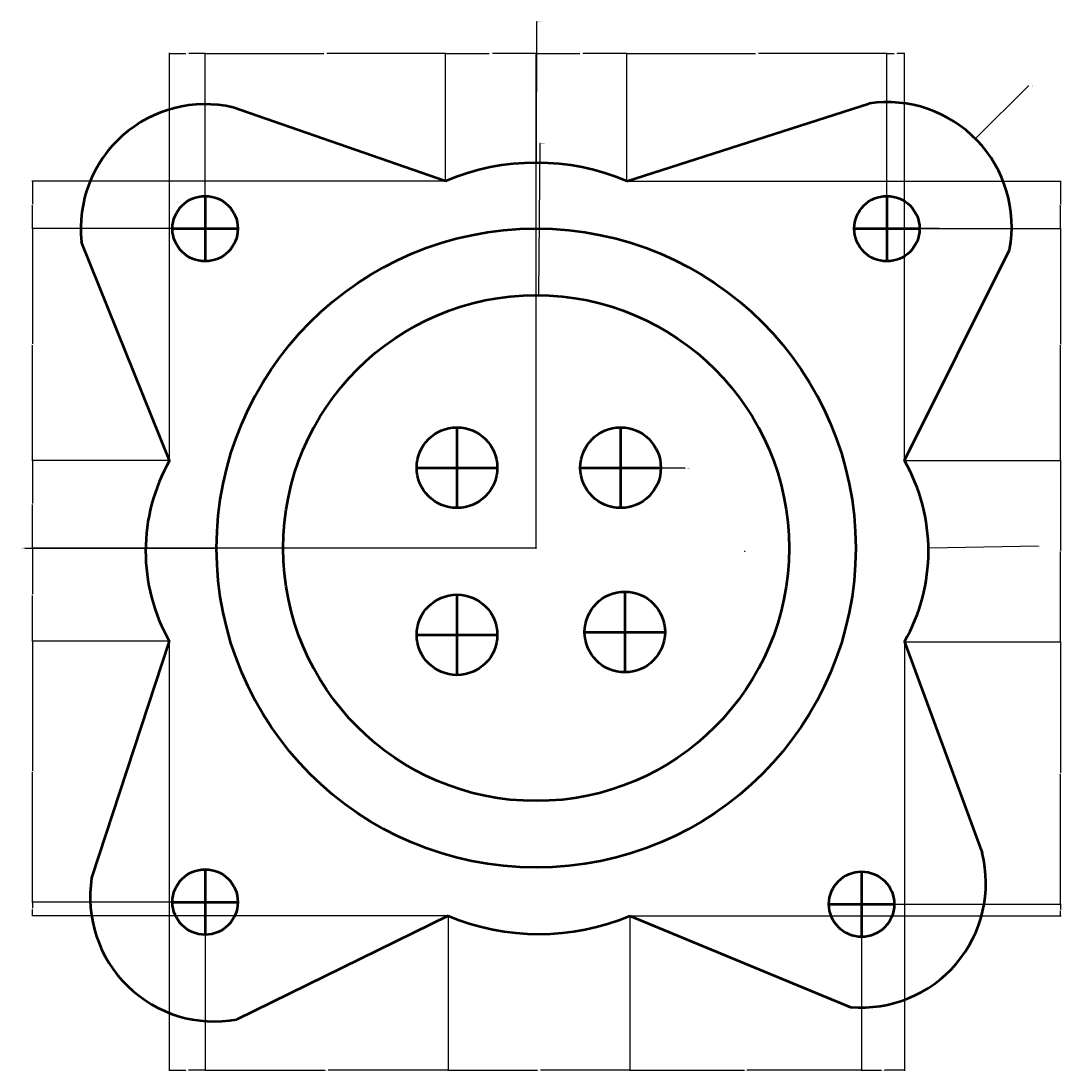
# Model space of a CAD drawing. Units: millimetres. Extents: x 2637 to 3282, y 1554 to 2264.
# Tile 2 of 3: x 2637 to 2920, y 1979 to 2264. Entities that reach past the tile are written whole.
import ezdxf

# ---------------------------------------------------------------- set-up
doc = ezdxf.new("R2010")
doc.units = ezdxf.units.MM
doc.layers.add('M-DIMS', color=2, linetype='Continuous', lineweight=18)
doc.layers.add('M-OUTL', color=7, linetype='Continuous', lineweight=50)
doc.styles.get("Standard").update_dxf_attribs({"font": 'arial.ttf'})
doc.dimstyles.get("Standard").update_dxf_attribs({"dimtxt": 0.18, "dimasz": 0.18, "dimexe": 0.18, "dimexo": 0.0625, "dimgap": 0.09, "dimtad": 0, "dimtih": 1, "dimtoh": 1, "dimdec": 4, "dimzin": 0, "dimdsep": 46, "dimtxsty": 'Standard', "dimcen": 0.09, "dimadec": 0, "dimazin": 0, "dimtfac": 1, "dimtdec": 4, "dimtofl": 0, "dimtmove": 0, "dimatfit": 3, "dimfxl": 1, "dimtolj": 1, "dimtzin": 0, "dimarcsym": 0})

# ---------------------------------------------------------------- blocks, each defined once
blk = doc.blocks.new('HOLE-MOUNT')
for p, q in [((2687.26, 1774.45), (2687.26, 1792.24)), ((2696.16, 1783.35), (2678.37, 1783.35))]:
    blk.add_line(p, q)
blk.add_circle((2687.26, 1783.35), 8.89)
blk = doc.blocks.new('HOLE-CENTRE')
for p, q in [((2755.81, 1707.32), (2755.81, 1729.25)), ((2766.78, 1718.29), (2744.85, 1718.29))]:
    blk.add_line(p, q)
blk.add_circle((2755.81, 1718.29), 10.96)
blk = doc.blocks.new('*D3')
at = {"layer": 'Defpoints', "color": 0, "transparency": 16777216}
for p in [(2687.26, 2255.59), (2687.26, 2207.95), (2677.6, 2144.89)]:
    blk.add_point(p, dxfattribs=at)
at = {"layer": 'M-DIMS', "color": 0, "lineweight": -2, "transparency": 16777216}
for p, q in [((2677.6, 2144.96), (2677.6, 2255.77)), ((2677.78, 2255.59), (2682.04, 2255.59)), ((2687.08, 2255.59), (2682.83, 2255.59)), ((2687.26, 2208.01), (2687.26, 2255.77))]:
    blk.add_line(p, q, dxfattribs=at)
at = {"layer": 'M-DIMS', "color": 0, "transparency": 16777216}
for points in [[(2677.78, 2255.62), (2677.78, 2255.56), (2677.6, 2255.59)], [(2687.08, 2255.62), (2687.08, 2255.56), (2687.26, 2255.59)]]:
    blk.add_solid(points, dxfattribs=at)
at = {"layer": 'M-DIMS', "color": 0, "transparency": 16777216, "insert": (2682.43, 2255.59), "char_height": 0.18, "attachment_point": 5}
blk.add_mtext('\\A1;9.662', dxfattribs=at)
blk = doc.blocks.new('*D4')
at = {"layer": 'Defpoints', "color": 0, "transparency": 16777216}
for p in [(2752.65, 2255.59), (2752.65, 2220.91), (2687.26, 2207.95)]:
    blk.add_point(p, dxfattribs=at)
at = {"layer": 'M-DIMS', "color": 0, "lineweight": -2, "transparency": 16777216}
for p, q in [((2687.26, 2208.01), (2687.26, 2255.77)), ((2687.44, 2255.59), (2719.56, 2255.59)), ((2752.47, 2255.59), (2720.35, 2255.59)), ((2752.65, 2220.98), (2752.65, 2255.77))]:
    blk.add_line(p, q, dxfattribs=at)
at = {"layer": 'M-DIMS', "color": 0, "transparency": 16777216}
for points in [[(2687.44, 2255.62), (2687.44, 2255.56), (2687.26, 2255.59)], [(2752.47, 2255.62), (2752.47, 2255.56), (2752.65, 2255.59)]]:
    blk.add_solid(points, dxfattribs=at)
at = {"layer": 'M-DIMS', "color": 0, "transparency": 16777216, "insert": (2719.96, 2255.59), "char_height": 0.18, "attachment_point": 5}
blk.add_mtext('\\A1;65.39', dxfattribs=at)
blk = doc.blocks.new('*D5')
at = {"layer": 'Defpoints', "color": 0, "transparency": 16777216}
for p in [(2777.37, 2255.59), (2752.65, 2220.91), (2777.37, 2121.01)]:
    blk.add_point(p, dxfattribs=at)
at = {"layer": 'M-DIMS', "color": 0, "lineweight": -2, "transparency": 16777216}
for p, q in [((2752.65, 2220.98), (2752.65, 2255.77)), ((2752.83, 2255.59), (2764.54, 2255.59)), ((2777.19, 2255.59), (2765.47, 2255.59)), ((2777.37, 2121.07), (2777.37, 2255.77))]:
    blk.add_line(p, q, dxfattribs=at)
at = {"layer": 'M-DIMS', "color": 0, "transparency": 16777216}
for points in [[(2752.83, 2255.62), (2752.83, 2255.56), (2752.65, 2255.59)], [(2777.19, 2255.62), (2777.19, 2255.56), (2777.37, 2255.59)]]:
    blk.add_solid(points, dxfattribs=at)
at = {"layer": 'M-DIMS', "color": 0, "transparency": 16777216, "insert": (2765.01, 2255.59), "char_height": 0.18, "attachment_point": 5}
blk.add_mtext('\\A1;24.715', dxfattribs=at)
blk = doc.blocks.new('*D6')
at = {"layer": 'Defpoints', "color": 0, "transparency": 16777216}
for p in [(2802.08, 2255.59), (2802.08, 2220.91), (2777.37, 2121.01)]:
    blk.add_point(p, dxfattribs=at)
at = {"layer": 'M-DIMS', "color": 0, "lineweight": -2, "transparency": 16777216}
for p, q in [((2777.37, 2121.07), (2777.37, 2255.77)), ((2777.55, 2255.59), (2789.26, 2255.59)), ((2801.9, 2255.59), (2790.19, 2255.59)), ((2802.08, 2220.98), (2802.08, 2255.77))]:
    blk.add_line(p, q, dxfattribs=at)
at = {"layer": 'M-DIMS', "color": 0, "transparency": 16777216}
for points in [[(2777.55, 2255.62), (2777.55, 2255.56), (2777.37, 2255.59)], [(2801.9, 2255.62), (2801.9, 2255.56), (2802.08, 2255.59)]]:
    blk.add_solid(points, dxfattribs=at)
at = {"layer": 'M-DIMS', "color": 0, "transparency": 16777216, "insert": (2789.72, 2255.59), "char_height": 0.18, "attachment_point": 5}
blk.add_mtext('\\A1;24.715', dxfattribs=at)
blk = doc.blocks.new('*D7')
at = {"layer": 'Defpoints', "color": 0, "transparency": 16777216}
for p in [(2872.83, 2255.59), (2802.08, 2220.91), (2872.83, 2207.95)]:
    blk.add_point(p, dxfattribs=at)
at = {"layer": 'M-DIMS', "color": 0, "lineweight": -2, "transparency": 16777216}
for p, q in [((2802.08, 2220.98), (2802.08, 2255.77)), ((2802.26, 2255.59), (2837.06, 2255.59)), ((2872.65, 2255.59), (2837.85, 2255.59)), ((2872.83, 2208.01), (2872.83, 2255.77))]:
    blk.add_line(p, q, dxfattribs=at)
at = {"layer": 'M-DIMS', "color": 0, "transparency": 16777216}
for points in [[(2802.26, 2255.62), (2802.26, 2255.56), (2802.08, 2255.59)], [(2872.65, 2255.62), (2872.65, 2255.56), (2872.83, 2255.59)]]:
    blk.add_solid(points, dxfattribs=at)
at = {"layer": 'M-DIMS', "color": 0, "transparency": 16777216, "insert": (2837.46, 2255.59), "char_height": 0.18, "attachment_point": 5}
blk.add_mtext('\\A1;70.75', dxfattribs=at)
blk = doc.blocks.new('*D8')
at = {"layer": 'Defpoints', "color": 0, "transparency": 16777216}
for p in [(2877.6, 2255.59), (2872.83, 2207.95), (2877.6, 2144.89)]:
    blk.add_point(p, dxfattribs=at)
at = {"layer": 'M-DIMS', "color": 0, "lineweight": -2, "transparency": 16777216}
for p, q in [((2872.83, 2208.01), (2872.83, 2255.77)), ((2873.01, 2255.59), (2874.82, 2255.59)), ((2877.42, 2255.59), (2875.62, 2255.59)), ((2877.6, 2144.96), (2877.6, 2255.77))]:
    blk.add_line(p, q, dxfattribs=at)
at = {"layer": 'M-DIMS', "color": 0, "transparency": 16777216}
for points in [[(2873.01, 2255.62), (2873.01, 2255.56), (2872.83, 2255.59)], [(2877.42, 2255.62), (2877.42, 2255.56), (2877.6, 2255.59)]]:
    blk.add_solid(points, dxfattribs=at)
at = {"layer": 'M-DIMS', "color": 0, "transparency": 16777216, "insert": (2875.22, 2255.59), "char_height": 0.18, "attachment_point": 5}
blk.add_mtext('\\A1;4.767', dxfattribs=at)
blk = doc.blocks.new('*D9')
at = {"layer": 'Defpoints', "color": 0, "transparency": 16777216}
for p in [(2677.5, 2095.64), (2687.26, 2024.68), (2687.26, 1978.87)]:
    blk.add_point(p, dxfattribs=at)
at = {"layer": 'M-DIMS', "color": 0, "lineweight": -2, "transparency": 16777216}
for p, q in [((2677.5, 2095.58), (2677.5, 1978.69)), ((2687.26, 2024.62), (2687.26, 1978.69)), ((2677.68, 1978.87), (2681.99, 1978.87)), ((2687.08, 1978.87), (2682.78, 1978.87))]:
    blk.add_line(p, q, dxfattribs=at)
at = {"layer": 'M-DIMS', "color": 0, "transparency": 16777216}
for points in [[(2677.68, 1978.9), (2677.68, 1978.84), (2677.5, 1978.87)], [(2687.08, 1978.9), (2687.08, 1978.84), (2687.26, 1978.87)]]:
    blk.add_solid(points, dxfattribs=at)
at = {"layer": 'M-DIMS', "color": 0, "transparency": 16777216, "insert": (2682.38, 1978.87), "char_height": 0.18, "attachment_point": 5}
blk.add_mtext('\\A1;9.765', dxfattribs=at)
blk = doc.blocks.new('*D10')
at = {"layer": 'Defpoints', "color": 0, "transparency": 16777216}
for p in [(2687.26, 2024.68), (2753.41, 2020.91), (2753.41, 1978.87)]:
    blk.add_point(p, dxfattribs=at)
at = {"layer": 'M-DIMS', "color": 0, "lineweight": -2, "transparency": 16777216}
for p, q in [((2687.26, 2024.62), (2687.26, 1978.69)), ((2753.41, 2020.85), (2753.41, 1978.69)), ((2687.44, 1978.87), (2719.94, 1978.87)), ((2753.23, 1978.87), (2720.73, 1978.87))]:
    blk.add_line(p, q, dxfattribs=at)
at = {"layer": 'M-DIMS', "color": 0, "transparency": 16777216}
for points in [[(2687.44, 1978.9), (2687.44, 1978.84), (2687.26, 1978.87)], [(2753.23, 1978.9), (2753.23, 1978.84), (2753.41, 1978.87)]]:
    blk.add_solid(points, dxfattribs=at)
at = {"layer": 'M-DIMS', "color": 0, "transparency": 16777216, "insert": (2720.34, 1978.87), "char_height": 0.18, "attachment_point": 5}
blk.add_mtext('\\A1;66.15', dxfattribs=at)
blk = doc.blocks.new('*D11')
at = {"layer": 'Defpoints', "color": 0, "transparency": 16777216}
for p in [(2753.41, 2020.91), (2802.84, 2020.91), (2802.84, 1978.87)]:
    blk.add_point(p, dxfattribs=at)
at = {"layer": 'M-DIMS', "color": 0, "lineweight": -2, "transparency": 16777216}
for p, q in [((2753.41, 2020.85), (2753.41, 1978.69)), ((2802.84, 2020.85), (2802.84, 1978.69)), ((2753.59, 1978.87), (2777.73, 1978.87)), ((2802.66, 1978.87), (2778.52, 1978.87))]:
    blk.add_line(p, q, dxfattribs=at)
at = {"layer": 'M-DIMS', "color": 0, "transparency": 16777216}
for points in [[(2753.59, 1978.9), (2753.59, 1978.84), (2753.41, 1978.87)], [(2802.66, 1978.9), (2802.66, 1978.84), (2802.84, 1978.87)]]:
    blk.add_solid(points, dxfattribs=at)
at = {"layer": 'M-DIMS', "color": 0, "transparency": 16777216, "insert": (2778.13, 1978.87), "char_height": 0.18, "attachment_point": 5}
blk.add_mtext('\\A1;49.43', dxfattribs=at)
blk = doc.blocks.new('*D12')
at = {"layer": 'Defpoints', "color": 0, "transparency": 16777216}
for p in [(2865.94, 2024.09), (2802.84, 2020.91), (2865.94, 1978.87)]:
    blk.add_point(p, dxfattribs=at)
at = {"layer": 'M-DIMS', "color": 0, "lineweight": -2, "transparency": 16777216}
for p, q in [((2865.94, 2024.02), (2865.94, 1978.69)), ((2802.84, 2020.85), (2802.84, 1978.69)), ((2803.02, 1978.87), (2834.08, 1978.87)), ((2865.76, 1978.87), (2834.7, 1978.87))]:
    blk.add_line(p, q, dxfattribs=at)
at = {"layer": 'M-DIMS', "color": 0, "transparency": 16777216}
for points in [[(2803.02, 1978.9), (2803.02, 1978.84), (2802.84, 1978.87)], [(2865.76, 1978.9), (2865.76, 1978.84), (2865.94, 1978.87)]]:
    blk.add_solid(points, dxfattribs=at)
at = {"layer": 'M-DIMS', "color": 0, "transparency": 16777216, "insert": (2834.39, 1978.87), "char_height": 0.18, "attachment_point": 5}
blk.add_mtext('\\A1;63.1', dxfattribs=at)
blk = doc.blocks.new('*D13')
at = {"layer": 'Defpoints', "color": 0, "transparency": 16777216}
for p in [(2877.6, 2095.46), (2865.94, 2024.09), (2877.6, 1978.87)]:
    blk.add_point(p, dxfattribs=at)
at = {"layer": 'M-DIMS', "color": 0, "lineweight": -2, "transparency": 16777216}
for p, q in [((2877.6, 2095.4), (2877.6, 1978.69)), ((2865.94, 2024.02), (2865.94, 1978.69)), ((2866.12, 1978.87), (2871.33, 1978.87)), ((2877.42, 1978.87), (2872.21, 1978.87))]:
    blk.add_line(p, q, dxfattribs=at)
at = {"layer": 'M-DIMS', "color": 0, "transparency": 16777216}
for points in [[(2866.12, 1978.9), (2866.12, 1978.84), (2865.94, 1978.87)], [(2877.42, 1978.9), (2877.42, 1978.84), (2877.6, 1978.87)]]:
    blk.add_solid(points, dxfattribs=at)
at = {"layer": 'M-DIMS', "color": 0, "transparency": 16777216, "insert": (2871.77, 1978.87), "char_height": 0.18, "attachment_point": 5}
blk.add_mtext('\\A1;11.661', dxfattribs=at)
blk = doc.blocks.new('*D14')
at = {"layer": 'Defpoints', "color": 0, "transparency": 16777216}
for p in [(2752.65, 2220.91), (2640.25, 2207.95), (2687.26, 2207.95)]:
    blk.add_point(p, dxfattribs=at)
at = {"layer": 'M-DIMS', "color": 0, "lineweight": -2, "transparency": 16777216}
for p, q in [((2752.59, 2220.91), (2640.07, 2220.91)), ((2640.25, 2220.73), (2640.25, 2214.61)), ((2640.25, 2208.13), (2640.25, 2214.25)), ((2687.2, 2207.95), (2640.07, 2207.95))]:
    blk.add_line(p, q, dxfattribs=at)
at = {"layer": 'M-DIMS', "color": 0, "transparency": 16777216}
for points in [[(2640.22, 2220.73), (2640.28, 2220.73), (2640.25, 2220.91)], [(2640.22, 2208.13), (2640.28, 2208.13), (2640.25, 2207.95)]]:
    blk.add_solid(points, dxfattribs=at)
at = {"layer": 'M-DIMS', "color": 0, "transparency": 16777216, "insert": (2640.25, 2214.43), "char_height": 0.18, "attachment_point": 5}
blk.add_mtext('\\A1;12.962', dxfattribs=at)
blk = doc.blocks.new('*D15')
at = {"layer": 'Defpoints', "color": 0, "transparency": 16777216}
for p in [(2687.26, 2207.95), (2640.25, 2144.89), (2677.6, 2144.89)]:
    blk.add_point(p, dxfattribs=at)
at = {"layer": 'M-DIMS', "color": 0, "lineweight": -2, "transparency": 16777216}
for p, q in [((2687.2, 2207.95), (2640.07, 2207.95)), ((2640.25, 2207.77), (2640.25, 2176.6)), ((2640.25, 2145.07), (2640.25, 2176.24)), ((2677.54, 2144.89), (2640.07, 2144.89))]:
    blk.add_line(p, q, dxfattribs=at)
at = {"layer": 'M-DIMS', "color": 0, "transparency": 16777216}
for points in [[(2640.22, 2207.77), (2640.28, 2207.77), (2640.25, 2207.95)], [(2640.22, 2145.07), (2640.28, 2145.07), (2640.25, 2144.89)]]:
    blk.add_solid(points, dxfattribs=at)
at = {"layer": 'M-DIMS', "color": 0, "transparency": 16777216, "insert": (2640.25, 2176.42), "char_height": 0.18, "attachment_point": 5}
blk.add_mtext('\\A1;63.06', dxfattribs=at)
blk = doc.blocks.new('*D16')
at = {"layer": 'Defpoints', "color": 0, "transparency": 16777216}
for p in [(2677.6, 2144.89), (2640.25, 2121.01), (2777.37, 2121.01)]:
    blk.add_point(p, dxfattribs=at)
at = {"layer": 'M-DIMS', "color": 0, "lineweight": -2, "transparency": 16777216}
for p, q in [((2677.54, 2144.89), (2640.07, 2144.89)), ((2640.25, 2144.71), (2640.25, 2133.13)), ((2640.25, 2121.19), (2640.25, 2132.77)), ((2777.3, 2121.01), (2640.07, 2121.01))]:
    blk.add_line(p, q, dxfattribs=at)
at = {"layer": 'M-DIMS', "color": 0, "transparency": 16777216}
for points in [[(2640.22, 2144.71), (2640.28, 2144.71), (2640.25, 2144.89)], [(2640.22, 2121.19), (2640.28, 2121.19), (2640.25, 2121.01)]]:
    blk.add_solid(points, dxfattribs=at)
at = {"layer": 'M-DIMS', "color": 0, "transparency": 16777216, "insert": (2640.25, 2132.95), "char_height": 0.18, "attachment_point": 5}
blk.add_mtext('\\A1;23.88', dxfattribs=at)
blk = doc.blocks.new('*D17')
at = {"layer": 'Defpoints', "color": 0, "transparency": 16777216}
for p in [(2777.37, 2121.01), (2640.25, 2095.64), (2677.5, 2095.64)]:
    blk.add_point(p, dxfattribs=at)
at = {"layer": 'M-DIMS', "color": 0, "lineweight": -2, "transparency": 16777216}
for p, q in [((2777.3, 2121.01), (2640.07, 2121.01)), ((2640.25, 2120.83), (2640.25, 2108.51)), ((2640.25, 2095.82), (2640.25, 2108.15)), ((2677.44, 2095.64), (2640.07, 2095.64))]:
    blk.add_line(p, q, dxfattribs=at)
at = {"layer": 'M-DIMS', "color": 0, "transparency": 16777216}
for points in [[(2640.22, 2120.83), (2640.28, 2120.83), (2640.25, 2121.01)], [(2640.22, 2095.82), (2640.28, 2095.82), (2640.25, 2095.64)]]:
    blk.add_solid(points, dxfattribs=at)
at = {"layer": 'M-DIMS', "color": 0, "transparency": 16777216, "insert": (2640.25, 2108.33), "char_height": 0.18, "attachment_point": 5}
blk.add_mtext('\\A1;25.37', dxfattribs=at)
blk = doc.blocks.new('*D18')
at = {"layer": 'Defpoints', "color": 0, "transparency": 16777216}
for p in [(2677.5, 2095.64), (2640.25, 2024.68), (2687.26, 2024.68)]:
    blk.add_point(p, dxfattribs=at)
at = {"layer": 'M-DIMS', "color": 0, "lineweight": -2, "transparency": 16777216}
for p, q in [((2677.44, 2095.64), (2640.07, 2095.64)), ((2640.25, 2095.46), (2640.25, 2060.35)), ((2640.25, 2024.86), (2640.25, 2059.98)), ((2687.2, 2024.68), (2640.07, 2024.68))]:
    blk.add_line(p, q, dxfattribs=at)
at = {"layer": 'M-DIMS', "color": 0, "transparency": 16777216}
for points in [[(2640.22, 2095.46), (2640.28, 2095.46), (2640.25, 2095.64)], [(2640.22, 2024.86), (2640.28, 2024.86), (2640.25, 2024.68)]]:
    blk.add_solid(points, dxfattribs=at)
at = {"layer": 'M-DIMS', "color": 0, "transparency": 16777216, "insert": (2640.25, 2060.16), "char_height": 0.18, "attachment_point": 5}
blk.add_mtext('\\A1;70.96', dxfattribs=at)
blk = doc.blocks.new('*D19')
at = {"layer": 'Defpoints', "color": 0, "transparency": 16777216}
for p in [(2687.26, 2024.68), (2640.25, 2020.91), (2753.41, 2020.91)]:
    blk.add_point(p, dxfattribs=at)
at = {"layer": 'M-DIMS', "color": 0, "lineweight": -2, "transparency": 16777216}
for p, q in [((2687.2, 2024.68), (2640.07, 2024.68)), ((2640.25, 2024.5), (2640.25, 2022.98)), ((2753.35, 2020.91), (2640.07, 2020.91)), ((2640.25, 2021.09), (2640.25, 2022.62))]:
    blk.add_line(p, q, dxfattribs=at)
at = {"layer": 'M-DIMS', "color": 0, "transparency": 16777216}
for points in [[(2640.22, 2024.5), (2640.28, 2024.5), (2640.25, 2024.68)], [(2640.22, 2021.09), (2640.28, 2021.09), (2640.25, 2020.91)]]:
    blk.add_solid(points, dxfattribs=at)
at = {"layer": 'M-DIMS', "color": 0, "transparency": 16777216, "insert": (2640.25, 2022.8), "char_height": 0.18, "attachment_point": 5}
blk.add_mtext('\\A1;3.77', dxfattribs=at)
blk = doc.blocks.new('*D20')
at = {"layer": 'Defpoints', "color": 0, "transparency": 16777216}
for p in [(2802.08, 2220.91), (2872.83, 2207.95), (2920.12, 2207.95)]:
    blk.add_point(p, dxfattribs=at)
at = {"layer": 'M-DIMS', "color": 0, "lineweight": -2, "transparency": 16777216}
for p, q in [((2802.14, 2220.91), (2920.3, 2220.91)), ((2920.12, 2220.73), (2920.12, 2214.61)), ((2920.12, 2208.13), (2920.12, 2214.25)), ((2872.9, 2207.95), (2920.3, 2207.95))]:
    blk.add_line(p, q, dxfattribs=at)
at = {"layer": 'M-DIMS', "color": 0, "transparency": 16777216}
for points in [[(2920.09, 2220.73), (2920.15, 2220.73), (2920.12, 2220.91)], [(2920.09, 2208.13), (2920.15, 2208.13), (2920.12, 2207.95)]]:
    blk.add_solid(points, dxfattribs=at)
at = {"layer": 'M-DIMS', "color": 0, "transparency": 16777216, "insert": (2920.12, 2214.43), "char_height": 0.18, "attachment_point": 5}
blk.add_mtext('\\A1;12.962', dxfattribs=at)
blk = doc.blocks.new('*D21')
at = {"layer": 'Defpoints', "color": 0, "transparency": 16777216}
for p in [(2872.83, 2207.95), (2877.6, 2144.89), (2920.12, 2144.89)]:
    blk.add_point(p, dxfattribs=at)
at = {"layer": 'M-DIMS', "color": 0, "lineweight": -2, "transparency": 16777216}
for p, q in [((2872.9, 2207.95), (2920.3, 2207.95)), ((2920.12, 2207.77), (2920.12, 2176.6)), ((2920.12, 2145.07), (2920.12, 2176.24)), ((2877.66, 2144.89), (2920.3, 2144.89))]:
    blk.add_line(p, q, dxfattribs=at)
at = {"layer": 'M-DIMS', "color": 0, "transparency": 16777216}
for points in [[(2920.09, 2207.77), (2920.15, 2207.77), (2920.12, 2207.95)], [(2920.09, 2145.07), (2920.15, 2145.07), (2920.12, 2144.89)]]:
    blk.add_solid(points, dxfattribs=at)
at = {"layer": 'M-DIMS', "color": 0, "transparency": 16777216, "insert": (2920.12, 2176.42), "char_height": 0.18, "attachment_point": 5}
blk.add_mtext('\\A1;63.06', dxfattribs=at)
blk = doc.blocks.new('*D22')
at = {"layer": 'Defpoints', "color": 0, "transparency": 16777216}
for p in [(2877.6, 2144.89), (2877.6, 2095.46), (2920.12, 2095.46)]:
    blk.add_point(p, dxfattribs=at)
at = {"layer": 'M-DIMS', "color": 0, "lineweight": -2, "transparency": 16777216}
for p, q in [((2877.66, 2144.89), (2920.3, 2144.89)), ((2920.12, 2144.71), (2920.12, 2120.36)), ((2920.12, 2095.64), (2920.12, 2120)), ((2877.66, 2095.46), (2920.3, 2095.46))]:
    blk.add_line(p, q, dxfattribs=at)
at = {"layer": 'M-DIMS', "color": 0, "transparency": 16777216}
for points in [[(2920.09, 2144.71), (2920.15, 2144.71), (2920.12, 2144.89)], [(2920.09, 2095.64), (2920.15, 2095.64), (2920.12, 2095.46)]]:
    blk.add_solid(points, dxfattribs=at)
at = {"layer": 'M-DIMS', "color": 0, "transparency": 16777216, "insert": (2920.12, 2120.18), "char_height": 0.18, "attachment_point": 5}
blk.add_mtext('\\A1;49.43', dxfattribs=at)
blk = doc.blocks.new('*D23')
at = {"layer": 'Defpoints', "color": 0, "transparency": 16777216}
for p in [(2877.6, 2095.46), (2865.94, 2024.09), (2920.12, 2024.09)]:
    blk.add_point(p, dxfattribs=at)
at = {"layer": 'M-DIMS', "color": 0, "lineweight": -2, "transparency": 16777216}
for p, q in [((2877.66, 2095.46), (2920.3, 2095.46)), ((2920.12, 2095.28), (2920.12, 2059.96)), ((2920.12, 2024.27), (2920.12, 2059.59)), ((2866, 2024.09), (2920.3, 2024.09))]:
    blk.add_line(p, q, dxfattribs=at)
at = {"layer": 'M-DIMS', "color": 0, "transparency": 16777216}
for points in [[(2920.09, 2095.28), (2920.15, 2095.28), (2920.12, 2095.46)], [(2920.09, 2024.27), (2920.15, 2024.27), (2920.12, 2024.09)]]:
    blk.add_solid(points, dxfattribs=at)
at = {"layer": 'M-DIMS', "color": 0, "transparency": 16777216, "insert": (2920.12, 2059.77), "char_height": 0.18, "attachment_point": 5}
blk.add_mtext('\\A1;71.38', dxfattribs=at)
blk = doc.blocks.new('*D24')
at = {"layer": 'Defpoints', "color": 0, "transparency": 16777216}
for p in [(2865.94, 2024.09), (2802.84, 2020.91), (2920.12, 2020.91)]:
    blk.add_point(p, dxfattribs=at)
at = {"layer": 'M-DIMS', "color": 0, "lineweight": -2, "transparency": 16777216}
for p, q in [((2866, 2024.09), (2920.3, 2024.09)), ((2920.12, 2023.91), (2920.12, 2022.68)), ((2802.9, 2020.91), (2920.3, 2020.91)), ((2920.12, 2021.09), (2920.12, 2022.32))]:
    blk.add_line(p, q, dxfattribs=at)
at = {"layer": 'M-DIMS', "color": 0, "transparency": 16777216}
for points in [[(2920.09, 2023.91), (2920.15, 2023.91), (2920.12, 2024.09)], [(2920.09, 2021.09), (2920.15, 2021.09), (2920.12, 2020.91)]]:
    blk.add_solid(points, dxfattribs=at)
at = {"layer": 'M-DIMS', "color": 0, "transparency": 16777216, "insert": (2920.12, 2022.5), "char_height": 0.18, "attachment_point": 5}
blk.add_mtext('\\A1;3.172', dxfattribs=at)
blk = doc.blocks.new('*D62')
at = {"layer": 'Defpoints', "color": 0, "transparency": 16777216}
for p in [(2690.39, 2121), (2864.34, 2121.02)]:
    blk.add_point(p, dxfattribs=at)
at = {"layer": 'M-DIMS', "color": 0, "lineweight": -2, "transparency": 16777216}
for p, q in [((2638.2, 2120.99), (2690.21, 2121)), ((2777.28, 2121.01), (2777.46, 2121.01)), ((2777.37, 2120.92), (2777.37, 2121.1))]:
    blk.add_line(p, q, dxfattribs=at)
at = {"layer": 'M-DIMS', "color": 0, "transparency": 16777216}
blk.add_solid([(2690.21, 2121.03), (2690.21, 2120.97), (2690.39, 2121)], dxfattribs=at)
at = {"layer": 'M-DIMS', "color": 0, "transparency": 16777216, "insert": (2637.64, 2120.99), "char_height": 0.18, "attachment_point": 5}
blk.add_mtext('\\A1;∅173.96', dxfattribs=at)
blk = doc.blocks.new('*D63')
at = {"layer": 'Defpoints', "color": 0, "transparency": 16777216}
for p in [(2778, 2189.84), (2776.73, 2052.18)]:
    blk.add_point(p, dxfattribs=at)
at = {"layer": 'M-DIMS', "color": 0, "lineweight": -2, "transparency": 16777216}
for p, q in [((2778.38, 2231.14), (2778, 2190.02)), ((2778.56, 2231.14), (2778.38, 2231.14)), ((2777.28, 2121.01), (2777.46, 2121.01)), ((2777.37, 2120.92), (2777.37, 2121.1))]:
    blk.add_line(p, q, dxfattribs=at)
at = {"layer": 'M-DIMS', "color": 0, "transparency": 16777216}
blk.add_solid([(2777.97, 2190.02), (2778.03, 2190.02), (2778, 2189.84)], dxfattribs=at)
at = {"layer": 'M-DIMS', "color": 0, "transparency": 16777216, "insert": (2779.12, 2231.14), "char_height": 0.18, "attachment_point": 5}
blk.add_mtext('\\A1;∅137.67', dxfattribs=at)
blk = doc.blocks.new('*D64')
at = {"layer": 'Defpoints', "color": 0, "transparency": 16777216}
for p in [(2789.37, 2142.98), (2811.3, 2142.8)]:
    blk.add_point(p, dxfattribs=at)
at = {"layer": 'M-DIMS', "color": 0, "lineweight": -2, "transparency": 16777216}
for p, q in [((2800.25, 2142.89), (2800.43, 2142.89)), ((2800.34, 2142.8), (2800.34, 2142.98)), ((2817.88, 2142.75), (2811.48, 2142.8))]:
    blk.add_line(p, q, dxfattribs=at)
at = {"layer": 'M-DIMS', "color": 0, "transparency": 16777216}
blk.add_solid([(2811.48, 2142.83), (2811.48, 2142.77), (2811.3, 2142.8)], dxfattribs=at)
at = {"layer": 'M-DIMS', "color": 0, "transparency": 16777216, "insert": (2818.56, 2142.75), "char_height": 0.18, "attachment_point": 5}
blk.add_mtext('\\A1;4X ∅21.93', dxfattribs=at)
blk = doc.blocks.new('*D65')
at = {"layer": 'Defpoints', "color": 0, "transparency": 16777216}
for p in [(2863.94, 2207.9), (2881.73, 2208)]:
    blk.add_point(p, dxfattribs=at)
at = {"layer": 'M-DIMS', "color": 0, "lineweight": -2, "transparency": 16777216}
for p, q in [((2872.74, 2207.95), (2872.92, 2207.95)), ((2872.83, 2207.86), (2872.83, 2208.04)), ((2887.06, 2208.03), (2881.91, 2208))]:
    blk.add_line(p, q, dxfattribs=at)
at = {"layer": 'M-DIMS', "color": 0, "transparency": 16777216}
blk.add_solid([(2881.91, 2208.03), (2881.91, 2207.97), (2881.73, 2208)], dxfattribs=at)
at = {"layer": 'M-DIMS', "color": 0, "transparency": 16777216, "insert": (2887.82, 2208.03), "char_height": 0.18, "attachment_point": 5}
blk.add_mtext('\\A1;4X ∅17.787', dxfattribs=at)
blk = doc.blocks.new('*D66')
at = {"layer": 'Defpoints', "color": 0, "transparency": 16777216}
for p in [(2896.93, 2232.43), (2872.96, 2208.52)]:
    blk.add_point(p, dxfattribs=at)
at = {"layer": 'M-DIMS', "color": 0, "lineweight": -2, "transparency": 16777216}
for p, q in [((2911.32, 2246.78), (2897.06, 2232.56)), ((2911.5, 2246.78), (2911.32, 2246.78)), ((2872.87, 2208.52), (2873.05, 2208.52)), ((2872.96, 2208.43), (2872.96, 2208.61))]:
    blk.add_line(p, q, dxfattribs=at)
at = {"layer": 'M-DIMS', "color": 0, "transparency": 16777216}
blk.add_solid([(2897.04, 2232.58), (2897.08, 2232.54), (2896.93, 2232.43)], dxfattribs=at)
at = {"layer": 'M-DIMS', "color": 0, "transparency": 16777216, "insert": (2912.17, 2246.78), "char_height": 0.18, "attachment_point": 5}
blk.add_mtext('\\A1;4X R33.86', dxfattribs=at)
blk = doc.blocks.new('*D67')
at = {"layer": 'Defpoints', "color": 0, "transparency": 16777216}
for p in [(2777.4, 2225.89), (2777.37, 2162.03)]:
    blk.add_point(p, dxfattribs=at)
at = {"layer": 'M-DIMS', "color": 0, "lineweight": -2, "transparency": 16777216}
for p, q in [((2777.42, 2264.2), (2777.4, 2226.07)), ((2777.6, 2264.2), (2777.42, 2264.2)), ((2777.28, 2162.03), (2777.46, 2162.03)), ((2777.37, 2161.94), (2777.37, 2162.12))]:
    blk.add_line(p, q, dxfattribs=at)
at = {"layer": 'M-DIMS', "color": 0, "transparency": 16777216}
blk.add_solid([(2777.37, 2226.07), (2777.43, 2226.07), (2777.4, 2225.89)], dxfattribs=at)
at = {"layer": 'M-DIMS', "color": 0, "transparency": 16777216, "insert": (2778.27, 2264.2), "char_height": 0.18, "attachment_point": 5}
blk.add_mtext('\\A1;2X R63.86', dxfattribs=at)
blk = doc.blocks.new('*D68')
at = {"layer": 'Defpoints', "color": 0, "transparency": 16777216}
for p in [(2884.14, 2121), (2834.19, 2120.18)]:
    blk.add_point(p, dxfattribs=at)
at = {"layer": 'M-DIMS', "color": 0, "lineweight": -2, "transparency": 16777216}
for p, q in [((2914.11, 2121.49), (2884.32, 2121)), ((2834.1, 2120.18), (2834.28, 2120.18)), ((2834.19, 2120.09), (2834.19, 2120.27))]:
    blk.add_line(p, q, dxfattribs=at)
at = {"layer": 'M-DIMS', "color": 0, "transparency": 16777216}
blk.add_solid([(2884.32, 2121.03), (2884.32, 2120.97), (2884.14, 2121)], dxfattribs=at)
at = {"layer": 'M-DIMS', "color": 0, "transparency": 16777216, "insert": (2914.78, 2121.49), "char_height": 0.18, "attachment_point": 5}
blk.add_mtext('\\A1;2X R49.95', dxfattribs=at)

msp = doc.modelspace()

# ---------------------------------------------------------------- linework, layer by layer
at = {"layer": 'M-OUTL'}
for p, q in [((2752.6515, 2220.913), (2694.8776, 2240.9462)), ((2802.0818, 2220.913), (2867.9757, 2242.0115)), ((2677.6018, 2144.893), (2653.599, 2204.3046)), ((2877.6018, 2144.893), (2906.2275, 2202.2205)), ((2677.4992, 2095.6442), (2656.3637, 2031.2404)), ((2877.6018, 2095.463), (2898.7651, 2038.0935)), ((2753.4101, 2020.913), (2695.8773, 1992.7022)), ((2802.8405, 2020.913), (2862.9407, 1996.1037))]:
    msp.add_line(p, q, dxfattribs=at)
for radius in [86.9781, 68.8327]:
    msp.add_circle((2777.3666, 2121.0119), radius, dxfattribs=at)
for centre, radius, start, end in [((2687.264, 2207.9514), 33.8619, 77.006317, 186.182441), ((2872.9563, 2208.5179), 33.8619, 349.282109, 98.458233), ((2777.3666, 2162.0338), 63.856, 67.229222, 112.770778), ((2777.3666, 2162.0338), 63.856, 67.229222, 112.770778), ((2721.0132, 2120.178), 49.9538, 150.346232, 209.414951), ((2834.1905, 2120.178), 49.9538, 330.346232, 29.653768), ((2865.926, 2029.8337), 33.8619, 264.94216, 14.118284), ((2689.8204, 2026.0179), 33.8619, 171.127908, 280.304032), ((2778.1253, 2079.7921), 63.856, 247.229222, 292.770778)]:
    msp.add_arc(centre, radius, start, end, dxfattribs=at)

# ---------------------------------------------------------------- block references
at = {"layer": 'M-OUTL', "rotation": 180}
for name, p in [('HOLE-MOUNT', (5374.5279, 3991.3)), ('HOLE-MOUNT', (5560.0987, 3991.3)), ('HOLE-CENTRE', (5511.6285, 3861.1759)), ('HOLE-CENTRE', (5556.1514, 3861.1759)), ('HOLE-CENTRE', (5557.3092, 3816.4593)), ('HOLE-CENTRE', (5511.6285, 3815.6885)), ('HOLE-MOUNT', (5374.5279, 3808.0315)), ('HOLE-MOUNT', (5553.2044, 3807.4338))]:
    msp.add_blockref(name, p, dxfattribs=at)

# ---------------------------------------------------------------- dimensions: what is measured, and where the dimension line sits
at = {"layer": 'M-DIMS'}
for center, mpoint, text, picture, middle in [((2777.3666, 2162.0338), (2777.4, 2225.8899), '2X <>', '*D67', (2778.2748, 2264.2035)), ((2872.9563, 2208.5179), (2896.9311, 2232.4311), '4X <>', '*D66', (2912.1728, 2246.7789)), ((2834.1905, 2120.178), (2884.1375, 2121.0006), '2X <>', '*D68', (2914.1056, 2121.4942))]:
    dim = msp.add_radius_dim(center=center, mpoint=mpoint, text=text, dimstyle='Standard', override={"dimdec": 2, "dimlfac": 1, "dimrnd": 0, "dimzin": 0, "dimdsep": 46, "dimlunit": 2}, dxfattribs=at)
    dim.commit()
    dim.dimension.update_dxf_attribs({"geometry": picture, "text_midpoint": middle, "dimtype": 164})
for base, p1, p2, override, picture, middle in [((2687.264, 2255.5864), (2677.6018, 2144.893), (2687.264, 2207.9514), {"dimdec": 3, "dimlfac": 1, "dimrnd": 0, "dimzin": 0, "dimdsep": 46, "dimlunit": 2}, '*D3', (2682.4329, 2255.5864)), ((2752.6515, 2255.5864), (2687.264, 2207.9514), (2752.6515, 2220.913), {"dimdec": 2, "dimlfac": 1, "dimrnd": 0, "dimzin": 0, "dimdsep": 46, "dimlunit": 2}, '*D4', (2719.9577, 2255.5864)), ((2777.3666, 2255.5864), (2752.6515, 2220.913), (2777.3666, 2121.0119), {"dimdec": 3, "dimlfac": 1, "dimrnd": 0, "dimzin": 0, "dimdsep": 46, "dimlunit": 2}, '*D5', (2765.0091, 2255.5864)), ((2802.0818, 2255.5864), (2777.3666, 2121.0119), (2802.0818, 2220.913), {"dimdec": 3, "dimlfac": 1, "dimrnd": 0, "dimzin": 0, "dimdsep": 46, "dimlunit": 2}, '*D6', (2789.7242, 2255.5864)), ((2872.8348, 2255.5864), (2802.0818, 2220.913), (2872.8348, 2207.9514), {"dimdec": 2, "dimlfac": 1, "dimrnd": 0, "dimzin": 0, "dimdsep": 46, "dimlunit": 2}, '*D7', (2837.4583, 2255.5864)), ((2877.6018, 2255.5864), (2872.8348, 2207.9514), (2877.6018, 2144.893), {"dimdec": 3, "dimlfac": 1, "dimrnd": 0, "dimzin": 0, "dimdsep": 46, "dimlunit": 2}, '*D8', (2875.2183, 2255.5864)), ((2687.264, 1978.8665), (2677.4992, 2095.6442), (2687.264, 2024.6828), {"dimdec": 3, "dimlfac": 1, "dimrnd": 0, "dimzin": 0, "dimdsep": 46, "dimlunit": 2}, '*D9', (2682.3816, 1978.8665)), ((2877.6018, 1978.8665), (2865.9404, 2024.0852), (2877.6018, 2095.463), {"dimdec": 3, "dimlfac": 1, "dimrnd": 0, "dimzin": 0, "dimdsep": 46, "dimlunit": 2}, '*D13', (2871.7711, 1978.8665)), ((2753.4101, 1978.8665), (2687.264, 2024.6828), (2753.4101, 2020.913), {"dimdec": 2, "dimlfac": 1, "dimrnd": 0, "dimzin": 0, "dimdsep": 46, "dimlunit": 2}, '*D10', (2720.3371, 1978.8665)), ((2865.9404, 1978.8665), (2802.8405, 2020.913), (2865.9404, 2024.0852), {"dimdec": 1, "dimlfac": 1, "dimrnd": 0, "dimzin": 0, "dimdsep": 46, "dimlunit": 2}, '*D12', (2834.3905, 1978.8665)), ((2802.8405, 1978.8665), (2753.4101, 2020.913), (2802.8405, 2020.913), {"dimdec": 2, "dimlfac": 1, "dimrnd": 0, "dimzin": 0, "dimdsep": 46, "dimlunit": 2}, '*D11', (2778.1253, 1978.8665))]:
    dim = msp.add_linear_dim(base=base, p1=p1, p2=p2, dimstyle='Standard', override=override, dxfattribs=at)
    dim.commit()
    dim.dimension.update_dxf_attribs({"geometry": picture, "text_midpoint": middle})
for p1, p2, picture, middle in [((2776.7347, 2052.1821), (2777.9985, 2189.8417), '*D63', (2779.1192, 2231.1396)), ((2864.3447, 2121.024), (2690.3886, 2120.9999), '*D62', (2638.2017, 2120.9927))]:
    dim = msp.add_diameter_dim_2p(p1=p1, p2=p2, dimstyle='Standard', override={"dimdec": 2, "dimlfac": 1, "dimrnd": 0, "dimzin": 0, "dimdsep": 46, "dimlunit": 2}, dxfattribs=at)
    dim.commit()
    dim.dimension.update_dxf_attribs({"geometry": picture, "text_midpoint": middle, "dimtype": 163})
for base, p1, p2, override, picture, middle in [((2640.249, 2207.9514), (2752.6515, 2220.913), (2687.264, 2207.9514), {"dimdec": 3, "dimlfac": 1, "dimrnd": 0, "dimzin": 0, "dimdsep": 46, "dimlunit": 2}, '*D14', (2640.249, 2214.4322)), ((2920.1215, 2207.9514), (2802.0818, 2220.913), (2872.8348, 2207.9514), {"dimdec": 3, "dimlfac": 1, "dimrnd": 0, "dimzin": 0, "dimdsep": 46, "dimlunit": 2}, '*D20', (2920.1215, 2214.4322)), ((2640.249, 2144.893), (2687.264, 2207.9514), (2677.6018, 2144.893), {"dimdec": 2, "dimlfac": 1, "dimrnd": 0, "dimzin": 0, "dimdsep": 46, "dimlunit": 2}, '*D15', (2640.249, 2176.4222)), ((2920.1215, 2144.893), (2872.8348, 2207.9514), (2877.6018, 2144.893), {"dimdec": 2, "dimlfac": 1, "dimrnd": 0, "dimzin": 0, "dimdsep": 46, "dimlunit": 2}, '*D21', (2920.1215, 2176.4222)), ((2640.249, 2121.0119), (2677.6018, 2144.893), (2777.3666, 2121.0119), {"dimdec": 2, "dimlfac": 1, "dimrnd": 0, "dimzin": 0, "dimdsep": 46, "dimlunit": 2}, '*D16', (2640.249, 2132.9525)), ((2920.1215, 2095.463), (2877.6018, 2144.893), (2877.6018, 2095.463), {"dimdec": 2, "dimlfac": 1, "dimrnd": 0, "dimzin": 0, "dimdsep": 46, "dimlunit": 2}, '*D22', (2920.1215, 2120.178)), ((2640.249, 2095.6442), (2777.3666, 2121.0119), (2677.4992, 2095.6442), {"dimdec": 2, "dimlfac": 1, "dimrnd": 0, "dimzin": 0, "dimdsep": 46, "dimlunit": 2}, '*D17', (2640.249, 2108.328)), ((2640.249, 2024.6828), (2677.4992, 2095.6442), (2687.264, 2024.6828), {"dimdec": 2, "dimlfac": 1, "dimrnd": 0, "dimzin": 0, "dimdsep": 46, "dimlunit": 2}, '*D18', (2640.249, 2060.1635)), ((2920.1215, 2024.0852), (2877.6018, 2095.463), (2865.9404, 2024.0852), {"dimdec": 2, "dimlfac": 1, "dimrnd": 0, "dimzin": 0, "dimdsep": 46, "dimlunit": 2}, '*D23', (2920.1215, 2059.7741)), ((2640.249, 2020.913), (2687.264, 2024.6828), (2753.4101, 2020.913), {"dimdec": 2, "dimlfac": 1, "dimrnd": 0, "dimzin": 0, "dimdsep": 46, "dimlunit": 2}, '*D19', (2640.249, 2022.7979)), ((2920.1215, 2020.913), (2865.9404, 2024.0852), (2802.8405, 2020.913), {"dimdec": 3, "dimlfac": 1, "dimrnd": 0, "dimzin": 0, "dimdsep": 46, "dimlunit": 2}, '*D24', (2920.1215, 2022.4991))]:
    dim = msp.add_linear_dim(base=base, p1=p1, p2=p2, angle=90, dimstyle='Standard', override=override, dxfattribs=at)
    dim.commit()
    dim.dimension.update_dxf_attribs({"geometry": picture, "text_midpoint": middle})
for p1, p2, override, picture, middle in [((2863.9412, 2207.9026), (2881.7283, 2208.0002), {"dimdec": 3, "dimlfac": 1, "dimrnd": 0, "dimzin": 0, "dimdsep": 46, "dimlunit": 2}, '*D65', (2887.0645, 2208.0294)), ((2789.3729, 2142.9795), (2811.3013, 2142.7992), {"dimdec": 2, "dimlfac": 1, "dimrnd": 0, "dimzin": 0, "dimdsep": 46, "dimlunit": 2}, '*D64', (2817.8799, 2142.7451))]:
    dim = msp.add_diameter_dim_2p(p1=p1, p2=p2, text='4X <>', dimstyle='Standard', override=override, dxfattribs=at)
    dim.commit()
    dim.dimension.update_dxf_attribs({"geometry": picture, "text_midpoint": middle, "dimtype": 163})

doc.saveas('drawing.dxf')
